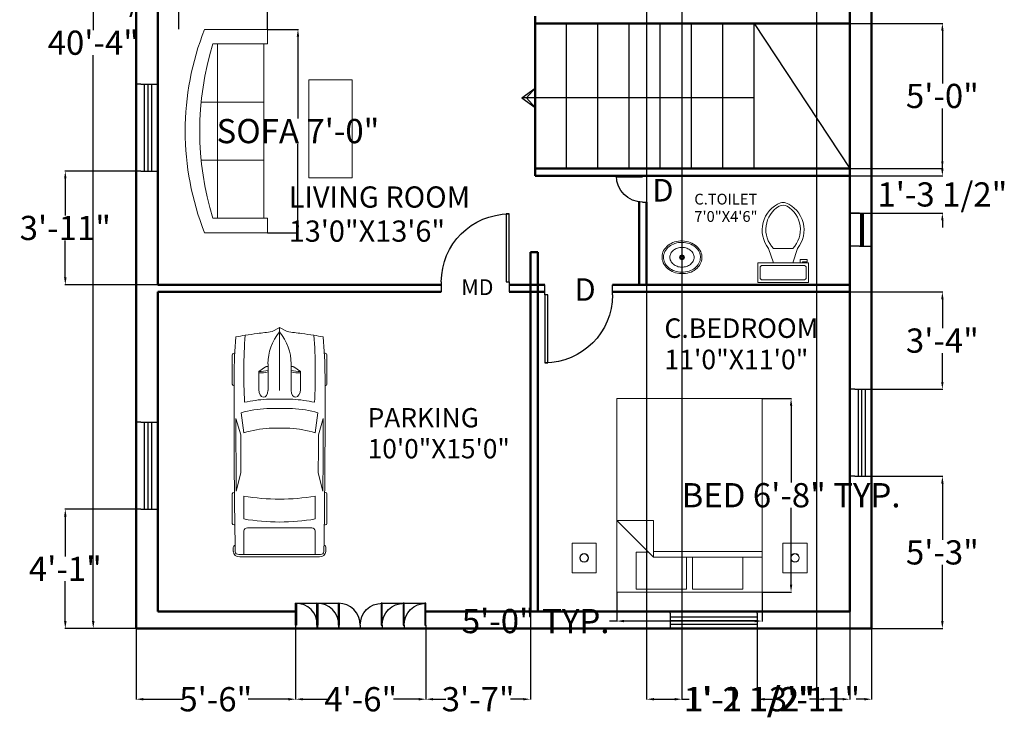
# Model space of a CAD drawing. Units: inches. Extents: x -35 to 382, y 867 to 1468.
# Tile 1 of 3: x -35 to 372, y 867 to 1163. Entities that reach past the tile are written whole.
import ezdxf

# ---------------------------------------------------------------- set-up
doc = ezdxf.new("R2010")
doc.units = ezdxf.units.IN
doc.header["$MEASUREMENT"] = 0
for name, color, linetype, lineweight in [('A-ANNO-DIMS', 2, 'Continuous', 18), ('A-ANNO-TEXT', 7, 'Continuous', 25), ('A-AREA-IDEN', 7, 'Continuous', 25), ('A-DOOR', 3, 'Continuous', 25), ('A-FLOR-FIXT', 9, 'Continuous', 18), ('A-FLOR-STRS', 7, 'Continuous', 25), ('A-FURN', 9, 'Continuous', 18), ('A-GLAZ', 4, 'Continuous', 25), ('A-SITE-VEHC', 8, 'Continuous', 13), ('A-WALL', 7, 'Continuous', 50)]:
    doc.layers.add(name, color=color, linetype=linetype, lineweight=lineweight)
doc.styles.get("Standard").update_dxf_attribs({"font": 'arial.ttf'})
doc.dimstyles.get("Standard").update_dxf_attribs({"dimtxt": 10, "dimasz": 3, "dimexe": 0.18, "dimexo": 0.0625, "dimgap": 0.09, "dimtad": 0, "dimtih": 1, "dimtoh": 1, "dimdec": 0, "dimzin": 0, "dimdsep": 46, "dimlunit": 3, "dimtxsty": 'Standard', "dimcen": 0.09, "dimadec": 0, "dimazin": 0, "dimtfac": 1, "dimtdec": 0, "dimtofl": 0, "dimtmove": 0, "dimatfit": 3, "dimfxl": 1, "dimtolj": 1, "dimtzin": 0, "dimarcsym": 0})

# ---------------------------------------------------------------- blocks, each defined once
blk = doc.blocks.new('Sofa - Roundback 7 ft.')
for p, q in [((-12.00002, -32.4421), (-12.00003, -6.5971)), ((11.99997, -32.4421), (11.99998, -6.5971)), ((-36.000027, -34), (-36.000027, -11.4696)), ((35.99998, -34), (35.99998, -11.4696)), ((-35.999844, -13.3819), (35.9998, -13.3819)), ((-36.000027, -32.4421), (35.99998, -32.4421))]:
    blk.add_line(p, q)
for points in [[(-36.000027, -34), (-42.000027, -34), (-42.000027, -8)], [(41.99998, -8), (41.99998, -34), (35.99998, -34)]]:
    blk.add_lwpolyline(points)
for centre, radius, start, end in [((0, -114.25), 114.25, 68.43141, 111.5686), ((-0.00001, -127.1968), 121.1968, 72.72033, 107.2797)]:
    blk.add_arc(centre, radius, start, end)
blk = doc.blocks.new('*U11')
for p, q in [((536, 950), (536, 936)), ((1182, 988), (568, 988)), ((1214, 950), (1214, 950)), ((2235, 810), (1899, 912)), ((3412, 904), (3030, 807)), ((3440, 942), (3440, 950)), ((3472, 988), (4087, 988)), ((4119, 950), (4119, 934)), ((4736, -851), (4736, 851)), ((4785, -832), (4785, 832)), ((1779, 801), (2195, 746)), ((3516, 746), (3994, 746)), ((4179, 670), (4179, -670)), ((4736, 746), (4242, 746)), ((820, 295), (918, 436)), ((918, 436), (1294, 436)), ((756, 241), (1313, 241)), ((816, 241), (816, 283)), ((1496, -274), (1496, 274)), ((1690, -267), (1690, 267)), ((2102, 216), (2102, -216)), ((4736, -267), (4736, 267)), ((83, 156), (3, 10)), ((0, 0), (1313, 0)), ((3, -10), (83, -156)), ((756, -241), (1313, -241)), ((816, -241), (816, -283)), ((820, -295), (918, -436)), ((918, -436), (1294, -436)), ((2195, -746), (1779, -801)), ((2235, -810), (1899, -912)), ((3412, -904), (3030, -807)), ((3994, -746), (3516, -746)), ((4242, -746), (4736, -746)), ((536, -950), (536, -936)), ((1182, -988), (568, -988)), ((1214, -950), (1214, -950)), ((3440, -942), (3440, -950)), ((3472, -988), (4087, -988)), ((4119, -950), (4119, -934))]:
    blk.add_line(p, q)
for centre, major_axis, ratio, start_param, end_param in [((6757, -699), (0, 7958), 0.842304, 1.367076, 1.39176), ((1046, -12468), (0, 13417), 0.842304, 0.00281, 0.075598), ((568, 950), (0, -37.6), 0.842304, 3.141593, 4.712389), ((1638, -268113), (0, 269063), 0.842304, -0.013397, 0.002797), ((1182, 950), (0, 37.6), 0.842304, -1.570796, 0), ((1638, -268113), (0, -269025), 0.842304, 3.133765, 3.140441), ((3472, 950), (0, -37.6), 0.842304, 3.141593, 4.712389), ((4087, 950), (0, 37.6), 0.842304, -1.570796, 0), ((4588, 910), (0, 56.4), 0.842304, -0.013017, 1.249894), ((1638, -268131), (0, 269121), 0.842304, -0.013397, -0.013017), ((4673, 851), (0, -75.2), 0.842304, 1.570796, 3.128196), ((4673, 832), (0, -133), 0.842304, 1.570796, 3.128196), ((6583, -699), (0, -7755), 0.842304, 4.528606, 4.561838), ((952, -15087), (0, -15833), 0.842304, 3.096046, 3.200911), ((3414, 137), (0, -2280), 0.842304, 4.449482, 4.652344), ((3436, 137), (0, 2077), 0.842304, 1.245306, 1.50788), ((3800, 71), (0, -2021), 0.842304, 4.372215, 4.640744), ((2433, -93125), (0, -93935), 0.842304, 3.134049, 3.144098), ((434, 0), (0, 3734), 0.842304, 4.511394, 4.913384), ((912, 0), (0, 3734), 0.842304, 4.511394, 4.913384), ((4242, 670), (0, 75.2), 0.842304, 0, 1.570796), ((-5194, 1331), (0, -6374), 0.842304, 1.385369, 1.434372), ((331, 432), (0, 696), 0.842304, 4.435146, 4.718221), ((361, 432), (0, 696), 0.842304, 4.435146, 4.718221), ((1290, 339), (161, -9), 0.603834, -1.395552, 1.581315), ((756, -1185), (0, 1427), 0.842304, 0, 0.590319), ((832, 283), (0, 18.8), 0.842304, 0.879714, 1.570796), ((16, 0), (0, -18.8), 0.842304, 4.131459, 5.293319), ((-5194, -1331), (0, 6374), 0.842304, -1.434372, -1.385369), ((756, 1185), (0, 1427), 0.842304, 2.551274, 3.141593), ((832, -283), (0, -18.8), 0.842304, 4.712389, 5.403472), ((331, -432), (0, -696), 0.842304, 1.564964, 1.848039), ((361, -432), (0, -696), 0.842304, 1.564964, 1.848039), ((3414, -137), (0, -2280), 0.842304, -1.510751, -1.307889), ((3436, -137), (0, -2077), 0.842304, -1.50788, -1.245306), ((3800, -71), (0, -2021), 0.842304, -1.499151, -1.230623), ((6583, 699), (0, 7755), 0.842304, 1.721348, 1.754579), ((6757, 699), (0, 7958), 0.842304, 1.749832, 1.774517), ((952, 15087), (0, -15833), 0.842304, -0.059319, 0.045547), ((2433, 93125), (0, -93935), 0.842304, -0.002505, 0.007544), ((4242, -670), (0, -75.2), 0.842304, 4.712389, 6.283185), ((1046, 12468), (0, -13417), 0.842304, -0.075598, -0.00281), ((568, -950), (0, 37.6), 0.842304, 1.570796, 3.141593), ((1638, 268113), (0, 269063), 0.842304, 3.138796, 3.15499), ((1182, -950), (0, -37.6), 0.842304, 0, 1.570796), ((1638, 268113), (0, -269025), 0.842304, 0.001152, 0.007828), ((3472, -950), (0, -37.6), 0.842304, -1.570796, 0), ((4087, -950), (0, 37.6), 0.842304, 3.141593, 4.712389), ((4588, -910), (0, -56.4), 0.842304, -1.249894, 0.013017), ((1638, 268131), (0, 269121), 0.842304, 3.15461, 3.15499), ((4673, -851), (0, 75.2), 0.842304, 3.15499, 4.712389), ((4673, -832), (0, -133), 0.842304, 0.013397, 1.570796)]:
    blk.add_ellipse(centre, major_axis=major_axis, ratio=ratio, start_param=start_param, end_param=end_param)
at = {"extrusion": (0, 0, -1)}
blk.add_ellipse((1290, -339), major_axis=(161, 9), ratio=0.603834, start_param=-1.395552, end_param=1.581315, dxfattribs=at)
blk = doc.blocks.new('*U9')
for p, q in [((0, 0), (0, -6)), ((40, 0), (40, -6))]:
    blk.add_line(p, q)
blk.add_lwpolyline([(0, 0), (0, 40), (1.75, 40), (1.75, 0)], close=True)
blk.add_arc((0, 0), 40, 0, 90)
blk = doc.blocks.new('Bed - Queen')
for p, q in [((0, -80.00003), (0, 0)), ((0, 0), (59.99999, 0)), ((59.99999, 0), (59.99999, -80.00003)), ((7.99999, -1.2), (28.79998, -1.2)), ((7.99999, -14.4), (7.99999, -1.2)), ((28.79998, -1.2), (28.79998, -14.4)), ((31.19999, -1.2), (51.99999, -1.2)), ((31.19999, -14.4), (31.19999, -1.2)), ((51.99999, -1.2), (51.99999, -16.4)), ((0, -14.4), (44.8, -14.4)), ((59.99999, -29.6), (44.8, -14.4)), ((44.8, -14.4), (44.8, -29.6)), ((44.8, -16.8), (0, -16.8)), ((51.99999, -16.4), (46.79936, -16.4)), ((44.8, -29.6), (59.99999, -29.6)), ((59.99999, -80.00003), (0, -80.00003))]:
    blk.add_line(p, q)
blk = doc.blocks.new('Sink - Oval top')
for p, q in [((-1, 0), (1, 0)), ((0, 1), (0, -1))]:
    blk.add_line(p, q)
for points in [[(-12.23, 0.39, 0.117634), (-11.46, -3.36, 0.104469), (-8.88, -6.8, 0.090016), (-5.08, -9.07, 0.08192), (-0.32, -10.02, 0.08192), (4.49, -9.38, 0.090016), (8.42, -7.36, 0.104469), (11.22, -4.09, 0.117634), (12.23, -0.39, 0.117634), (11.46, 3.36, 0.104469), (8.88, 6.8, 0.090016), (5.08, 9.07, 0.08192), (0.32, 10.02, 0.08192), (-4.49, 9.38, 0.090016), (-8.42, 7.36, 0.104469), (-11.22, 4.09, 0.117634)], [(-11.29, 0.16, 0.118622), (-10.52, -3.25, 0.104678), (-8.07, -6.36, 0.089562), (-4.54, -8.37, 0.081185), (-0.13, -9.15, 0.081185), (4.3, -8.49, 0.089562), (7.89, -6.58, 0.104678), (10.42, -3.55, 0.118622), (11.29, -0.16, 0.118622), (10.52, 3.25, 0.104678), (8.07, 6.36, 0.089562), (4.54, 8.37, 0.081185), (0.13, 9.15, 0.081185), (-4.3, 8.49, 0.089562), (-7.89, 6.58, 0.104678), (-10.42, 3.55, 0.118622)], [(-7.42, 0.08, 0.118283), (-6.91, -2.17, 0.104607), (-5.29, -4.21, 0.089718), (-2.97, -5.53, 0.081436), (-0.07, -6.04, 0.081436), (2.84, -5.59, 0.089718), (5.2, -4.33, 0.104607), (6.86, -2.32, 0.118283), (7.42, -0.08, 0.118283), (6.91, 2.17, 0.104607), (5.29, 4.21, 0.089718), (2.97, 5.53, 0.081436), (0.07, 6.04, 0.081436), (-2.84, 5.59, 0.089718), (-5.2, 4.33, 0.104607), (-6.86, 2.32, 0.118283)]]:
    blk.add_lwpolyline(points, format="xyb", close=True)
for radius in [1.5, 1]:
    blk.add_circle((0, 0), radius)
blk = doc.blocks.new('Toilet - top')
for p, q in [((9.5, -6), (9.5, -2)), ((-8, -8.5), (-8, -8)), ((-7, -8), (-7, -9.5)), ((-4, -8), (-6, -14)), ((4, -8), (6, -14)), ((-10, -8.5), (-8, -8.5)), ((-10, -9.5), (-10, -8.5)), ((-7, -9.5), (-10, -9.5)), ((4, -14), (-4, -14))]:
    blk.add_line(p, q)
blk.add_lwpolyline([(10.5, -8), (10.5, 0), (-10.5, 0), (-10.5, -8)], close=True)
for points in [[(-9.5, -2), (-9.5, -6)], [(8.5, -1), (-8.5, -1)], [(-8.5, -7), (8.5, -7)]]:
    blk.add_lwpolyline(points)
for centre, radius, start, end in [((-8.62, -1.88), 0.884, 81.8699, 188.1301), ((8.62, -1.88), 0.884, 351.8699, 98.1301), ((-8.62, -6.12), 0.884, 171.8699, 278.1301), ((8.62, -6.12), 0.884, 261.8699, 8.1301), ((3.52, -21.58), 12.17, 141.4691, 247.9714), ((4.2, -21.82), 11.33, 136.3677, 238.9468), ((-3.52, -21.58), 12.17, 292.0284, 38.5307), ((-4.2, -21.82), 11.33, 301.053, 43.6321), ((0, -27.88), 4, 245.7318, 294.2682), ((0, -29), 4, 254.8605, 285.1395)]:
    blk.add_arc(centre, radius, start, end)
blk = doc.blocks.new('Window - Wood Frame 36 in. Wide plan')
for p, q in [((0, 6), (0, 0)), ((0, 4.5), (36, 4.5)), ((36, 6), (36, 0)), ((0, 3), (36, 3)), ((0, 1.5), (36, 1.5))]:
    blk.add_line(p, q)
blk = doc.blocks.new('*D16')
at = {"layer": 'A-ANNO-DIMS', "color": 0, "lineweight": -2, "transparency": 16777216}
for p, q in [((13.46, 1395.31), (-4.36, 1395.31)), ((-4.18, 1392.31), (-4.18, 1158.51)), ((-4.18, 914.31), (-4.18, 1148.12)), ((13.46, 911.31), (-4.36, 911.31))]:
    blk.add_line(p, q, dxfattribs=at)
at = {"layer": 'A-ANNO-DIMS', "color": 0, "transparency": 16777216}
for points in [[(-4.68, 1392.31), (-3.68, 1392.31), (-4.18, 1395.31)], [(-4.68, 914.31), (-3.68, 914.31), (-4.18, 911.31)]]:
    blk.add_solid(points, dxfattribs=at)
at = {"layer": 'Defpoints', "color": 0, "transparency": 16777216}
for p in [(13.52, 1395.31), (-4.18, 911.31), (13.52, 911.31)]:
    blk.add_point(p, dxfattribs=at)
at = {"layer": 'A-ANNO-DIMS', "color": 0, "transparency": 16777216, "insert": (-4.18, 1153.31), "char_height": 10, "attachment_point": 5}
blk.add_mtext('\\A1;40\'-4"', dxfattribs=at)
blk = doc.blocks.new('BEDSIDE-TABLE')
blk.add_lwpolyline([(0, 12.34), (9.96, 12.34), (9.96, 0), (0, 0)], close=True)
for radius in [1.78, 1.78, 1.66]:
    blk.add_circle((4.98, 6.17), radius)
blk = doc.blocks.new('*D24')
at = {"layer": 'A-ANNO-DIMS', "color": 0, "lineweight": -2, "transparency": 16777216}
for p, q in [((272.3, 1006.35), (284.42, 1006.35)), ((284.24, 1003.35), (284.24, 971.55)), ((284.24, 929.35), (284.24, 961.16)), ((272.3, 926.35), (284.42, 926.35))]:
    blk.add_line(p, q, dxfattribs=at)
at = {"layer": 'A-ANNO-DIMS', "color": 0, "transparency": 16777216}
for points in [[(283.74, 1003.35), (284.74, 1003.35), (284.24, 1006.35)], [(283.74, 929.35), (284.74, 929.35), (284.24, 926.35)]]:
    blk.add_solid(points, dxfattribs=at)
at = {"layer": 'Defpoints', "color": 0, "transparency": 16777216}
for p in [(272.24, 1006.35), (272.24, 926.35), (284.24, 926.35)]:
    blk.add_point(p, dxfattribs=at)
at = {"layer": 'A-ANNO-DIMS', "color": 0, "transparency": 16777216, "insert": (284.24, 966.35), "char_height": 10, "attachment_point": 5}
blk.add_mtext('\\A1;BED 6\'-8" TYP.', dxfattribs=at)
blk = doc.blocks.new('*D25')
at = {"layer": 'A-ANNO-DIMS', "color": 0, "lineweight": -2, "transparency": 16777216}
for p, q in [((212.24, 926.29), (212.24, 914.17)), ((272.24, 926.29), (272.24, 914.17)), ((212.24, 914.35), (209.24, 914.35)), ((269.24, 914.35), (215.24, 914.35))]:
    blk.add_line(p, q, dxfattribs=at)
at = {"layer": 'A-ANNO-DIMS', "color": 0, "transparency": 16777216}
for points in [[(215.24, 914.85), (215.24, 913.85), (212.24, 914.35)], [(269.24, 914.85), (269.24, 913.85), (272.24, 914.35)]]:
    blk.add_solid(points, dxfattribs=at)
at = {"layer": 'Defpoints', "color": 0, "transparency": 16777216}
for p in [(212.24, 926.35), (272.24, 926.35), (212.24, 914.35)]:
    blk.add_point(p, dxfattribs=at)
at = {"layer": 'A-ANNO-DIMS', "color": 0, "transparency": 16777216, "insert": (178.67, 914.35), "char_height": 10, "attachment_point": 5}
blk.add_mtext('\\A1;5\'-0" TYP.', dxfattribs=at)
blk = doc.blocks.new('*D30')
at = {"layer": 'A-ANNO-DIMS', "color": 0, "lineweight": -2, "transparency": 16777216}
for p, q in [((67.88, 1158.79), (80.6, 1158.79)), ((80.42, 1155.79), (80.42, 1122.05)), ((80.42, 1077.79), (80.42, 1111.52)), ((67.88, 1074.79), (80.6, 1074.79))]:
    blk.add_line(p, q, dxfattribs=at)
at = {"layer": 'A-ANNO-DIMS', "color": 0, "transparency": 16777216}
for points in [[(79.92, 1155.79), (80.92, 1155.79), (80.42, 1158.79)], [(79.92, 1077.79), (80.92, 1077.79), (80.42, 1074.79)]]:
    blk.add_solid(points, dxfattribs=at)
at = {"layer": 'Defpoints', "color": 0, "transparency": 16777216}
for p in [(67.82, 1158.79), (80.42, 1158.79), (67.82, 1074.79)]:
    blk.add_point(p, dxfattribs=at)
at = {"layer": 'A-ANNO-DIMS', "color": 0, "transparency": 16777216, "insert": (80.42, 1116.79), "char_height": 10, "attachment_point": 5}
blk.add_mtext('\\A1;SOFA 7\'-0"', dxfattribs=at)
blk = doc.blocks.new('*D31')
at = {"layer": 'A-ANNO-DIMS', "color": 0, "lineweight": -2, "transparency": 16777216}
for p, q in [((31.15, 1171.39), (28.15, 1171.39)), ((31.15, 1158.85), (31.15, 1171.57)), ((64.82, 1171.39), (34.15, 1171.39)), ((67.82, 1158.85), (67.82, 1171.57))]:
    blk.add_line(p, q, dxfattribs=at)
at = {"layer": 'A-ANNO-DIMS', "color": 0, "transparency": 16777216}
for points in [[(34.15, 1171.89), (34.15, 1170.89), (31.15, 1171.39)], [(64.82, 1171.89), (64.82, 1170.89), (67.82, 1171.39)]]:
    blk.add_solid(points, dxfattribs=at)
at = {"layer": 'Defpoints', "color": 0, "transparency": 16777216}
for p in [(31.15, 1171.39), (31.15, 1158.79), (67.82, 1158.79)]:
    blk.add_point(p, dxfattribs=at)
at = {"layer": 'A-ANNO-DIMS', "color": 0, "transparency": 16777216, "insert": (3.12, 1171.39), "char_height": 10, "attachment_point": 5}
blk.add_mtext('\\A1;3\'-0 1/2"', dxfattribs=at)
blk = doc.blocks.new('*D36')
at = {"layer": 'A-ANNO-DIMS', "color": 0, "lineweight": -2, "transparency": 16777216}
for p, q in [((87.91, 1187.13), (87.91, 1173.36)), ((178.91, 1187.13), (178.91, 1173.36)), ((90.91, 1173.54), (175.91, 1173.54)), ((178.91, 1173.54), (181.91, 1173.54))]:
    blk.add_line(p, q, dxfattribs=at)
at = {"layer": 'A-ANNO-DIMS', "color": 0, "transparency": 16777216}
for points in [[(90.91, 1174.04), (90.91, 1173.04), (87.91, 1173.54)], [(175.91, 1174.04), (175.91, 1173.04), (178.91, 1173.54)]]:
    blk.add_solid(points, dxfattribs=at)
at = {"layer": 'Defpoints', "color": 0, "transparency": 16777216}
for p in [(87.91, 1187.19), (178.91, 1187.19), (178.91, 1173.54)]:
    blk.add_point(p, dxfattribs=at)
at = {"layer": 'A-ANNO-DIMS', "color": 0, "transparency": 16777216, "insert": (236.96, 1173.54), "char_height": 10, "attachment_point": 5}
blk.add_mtext('\\A1;DINING SET 7\'-7"', dxfattribs=at)
blk = doc.blocks.new('*D38')
at = {"layer": 'A-ANNO-DIMS', "color": 0, "lineweight": -2, "transparency": 16777216}
for p, q in [((13.52, 911.25), (13.52, 881.88)), ((79.43, 911.25), (79.43, 881.88)), ((16.52, 882.06), (33.09, 882.06)), ((76.43, 882.06), (59.86, 882.06))]:
    blk.add_line(p, q, dxfattribs=at)
at = {"layer": 'A-ANNO-DIMS', "color": 0, "transparency": 16777216}
for points in [[(16.52, 882.56), (16.52, 881.56), (13.52, 882.06)], [(76.43, 882.56), (76.43, 881.56), (79.43, 882.06)]]:
    blk.add_solid(points, dxfattribs=at)
at = {"layer": 'Defpoints', "color": 0, "transparency": 16777216}
for p in [(13.52, 911.31), (79.43, 911.31), (79.43, 882.06)]:
    blk.add_point(p, dxfattribs=at)
at = {"layer": 'A-ANNO-DIMS', "color": 0, "transparency": 16777216, "insert": (46.47, 882.06), "char_height": 10, "attachment_point": 5}
blk.add_mtext('\\A1;5\'-6"', dxfattribs=at)
blk = doc.blocks.new('*D39')
at = {"layer": 'A-ANNO-DIMS', "color": 0, "lineweight": -2, "transparency": 16777216}
for p, q in [((79.43, 911.25), (79.43, 881.88)), ((133.31, 911.25), (133.31, 881.88)), ((82.43, 882.06), (92.78, 882.06)), ((130.31, 882.06), (119.95, 882.06))]:
    blk.add_line(p, q, dxfattribs=at)
at = {"layer": 'A-ANNO-DIMS', "color": 0, "transparency": 16777216}
for points in [[(82.43, 882.56), (82.43, 881.56), (79.43, 882.06)], [(130.31, 882.56), (130.31, 881.56), (133.31, 882.06)]]:
    blk.add_solid(points, dxfattribs=at)
at = {"layer": 'Defpoints', "color": 0, "transparency": 16777216}
for p in [(79.43, 911.31), (133.31, 911.31), (133.31, 882.06)]:
    blk.add_point(p, dxfattribs=at)
at = {"layer": 'A-ANNO-DIMS', "color": 0, "transparency": 16777216, "insert": (106.37, 882.06), "char_height": 10, "attachment_point": 5}
blk.add_mtext('\\A1;4\'-6"', dxfattribs=at)
blk = doc.blocks.new('*D40')
at = {"layer": 'A-ANNO-DIMS', "color": 0, "lineweight": -2, "transparency": 16777216}
for p, q in [((176.52, 918.25), (176.52, 881.88)), ((133.31, 911.25), (133.31, 881.88)), ((136.31, 882.06), (141.54, 882.06)), ((173.52, 882.06), (168.29, 882.06))]:
    blk.add_line(p, q, dxfattribs=at)
at = {"layer": 'A-ANNO-DIMS', "color": 0, "transparency": 16777216}
for points in [[(136.31, 882.56), (136.31, 881.56), (133.31, 882.06)], [(173.52, 882.56), (173.52, 881.56), (176.52, 882.06)]]:
    blk.add_solid(points, dxfattribs=at)
at = {"layer": 'Defpoints', "color": 0, "transparency": 16777216}
for p in [(176.52, 918.31), (133.31, 911.31), (176.52, 882.06)]:
    blk.add_point(p, dxfattribs=at)
at = {"layer": 'A-ANNO-DIMS', "color": 0, "transparency": 16777216, "insert": (154.91, 882.06), "char_height": 10, "attachment_point": 5}
blk.add_mtext('\\A1;3\'-7"', dxfattribs=at)
blk = doc.blocks.new('*D41')
at = {"layer": 'A-ANNO-DIMS', "color": 0, "lineweight": -2, "transparency": 16777216}
for p, q in [((270.28, 911.51), (270.28, 881.88)), ((317.52, 911.25), (317.52, 881.88)), ((273.28, 882.06), (276.64, 882.06)), ((314.52, 882.06), (311.17, 882.06))]:
    blk.add_line(p, q, dxfattribs=at)
at = {"layer": 'A-ANNO-DIMS', "color": 0, "transparency": 16777216}
for points in [[(273.28, 882.56), (273.28, 881.56), (270.28, 882.06)], [(314.52, 882.56), (314.52, 881.56), (317.52, 882.06)]]:
    blk.add_solid(points, dxfattribs=at)
at = {"layer": 'Defpoints', "color": 0, "transparency": 16777216}
for p in [(270.28, 911.57), (317.52, 911.31), (270.28, 882.06)]:
    blk.add_point(p, dxfattribs=at)
at = {"layer": 'A-ANNO-DIMS', "color": 0, "transparency": 16777216, "insert": (293.9, 882.06), "char_height": 10, "attachment_point": 5}
blk.add_mtext('\\A1;3\'-11"', dxfattribs=at)
blk = doc.blocks.new('*D42')
at = {"layer": 'A-ANNO-DIMS', "color": 0, "lineweight": -2, "transparency": 16777216}
for p, q in [((308.58, 1050.31), (346.95, 1050.31)), ((346.77, 1047.31), (346.77, 1035.43)), ((346.77, 1013.15), (346.77, 1025.03)), ((317.58, 1010.15), (346.95, 1010.15))]:
    blk.add_line(p, q, dxfattribs=at)
at = {"layer": 'A-ANNO-DIMS', "color": 0, "transparency": 16777216}
for points in [[(346.27, 1047.31), (347.27, 1047.31), (346.77, 1050.31)], [(346.27, 1013.15), (347.27, 1013.15), (346.77, 1010.15)]]:
    blk.add_solid(points, dxfattribs=at)
at = {"layer": 'Defpoints', "color": 0, "transparency": 16777216}
for p in [(308.52, 1050.31), (346.77, 1050.31), (317.52, 1010.15)]:
    blk.add_point(p, dxfattribs=at)
at = {"layer": 'A-ANNO-DIMS', "color": 0, "transparency": 16777216, "insert": (346.77, 1030.23), "char_height": 10, "attachment_point": 5}
blk.add_mtext('\\A1;3\'-4"', dxfattribs=at)
blk = doc.blocks.new('*D44')
at = {"layer": 'A-ANNO-DIMS', "color": 0, "lineweight": -2, "transparency": 16777216}
for p, q in [((308.58, 1161.31), (346.95, 1161.31)), ((346.77, 1158.31), (346.77, 1136.51)), ((346.77, 1104.31), (346.77, 1126.12)), ((308.58, 1101.31), (346.95, 1101.31))]:
    blk.add_line(p, q, dxfattribs=at)
at = {"layer": 'A-ANNO-DIMS', "color": 0, "transparency": 16777216}
for points in [[(346.27, 1158.31), (347.27, 1158.31), (346.77, 1161.31)], [(346.27, 1104.31), (347.27, 1104.31), (346.77, 1101.31)]]:
    blk.add_solid(points, dxfattribs=at)
at = {"layer": 'Defpoints', "color": 0, "transparency": 16777216}
for p in [(308.52, 1161.31), (346.77, 1161.31), (308.52, 1101.31)]:
    blk.add_point(p, dxfattribs=at)
at = {"layer": 'A-ANNO-DIMS', "color": 0, "transparency": 16777216, "insert": (346.77, 1131.31), "char_height": 10, "attachment_point": 5}
blk.add_mtext('\\A1;5\'-0"', dxfattribs=at)
blk = doc.blocks.new('*D45')
at = {"layer": 'A-ANNO-DIMS', "color": 0, "lineweight": -2, "transparency": 16777216}
for p, q in [((239.15, 1224.59), (239.15, 881.88)), ((224.52, 1215.25), (224.52, 881.88)), ((227.52, 882.06), (236.15, 882.06)), ((239.15, 882.06), (242.15, 882.06))]:
    blk.add_line(p, q, dxfattribs=at)
at = {"layer": 'A-ANNO-DIMS', "color": 0, "transparency": 16777216}
for points in [[(227.52, 882.56), (227.52, 881.56), (224.52, 882.06)], [(236.15, 882.56), (236.15, 881.56), (239.15, 882.06)]]:
    blk.add_solid(points, dxfattribs=at)
at = {"layer": 'Defpoints', "color": 0, "transparency": 16777216}
for p in [(239.15, 1224.65), (224.52, 1215.31), (239.15, 882.06)]:
    blk.add_point(p, dxfattribs=at)
at = {"layer": 'A-ANNO-DIMS', "color": 0, "transparency": 16777216, "insert": (266.71, 882.06), "char_height": 10, "attachment_point": 5}
blk.add_mtext('\\A1;1\'-2 1/2"', dxfattribs=at)
blk = doc.blocks.new('*D46')
at = {"layer": 'A-ANNO-DIMS', "color": 0, "lineweight": -2, "transparency": 16777216}
for p, q in [((294.81, 1215.25), (294.81, 881.88)), ((308.52, 1215.25), (308.52, 881.88)), ((294.81, 882.06), (291.81, 882.06)), ((305.52, 882.06), (297.81, 882.06))]:
    blk.add_line(p, q, dxfattribs=at)
at = {"layer": 'A-ANNO-DIMS', "color": 0, "transparency": 16777216}
for points in [[(297.81, 882.56), (297.81, 881.56), (294.81, 882.06)], [(305.52, 882.56), (305.52, 881.56), (308.52, 882.06)]]:
    blk.add_solid(points, dxfattribs=at)
at = {"layer": 'Defpoints', "color": 0, "transparency": 16777216}
for p in [(294.81, 1215.31), (308.52, 1215.31), (294.81, 882.06)]:
    blk.add_point(p, dxfattribs=at)
at = {"layer": 'A-ANNO-DIMS', "color": 0, "transparency": 16777216, "insert": (267.25, 882.06), "char_height": 10, "attachment_point": 5}
blk.add_mtext('\\A1;1\'-1 1/2"', dxfattribs=at)
blk = doc.blocks.new('*D50')
at = {"layer": 'A-ANNO-DIMS', "color": 0, "lineweight": -2, "transparency": 16777216}
for p, q in [((317.58, 974.15), (346.95, 974.15)), ((346.77, 971.15), (346.77, 947.93)), ((346.77, 914.31), (346.77, 937.53)), ((317.58, 911.31), (346.95, 911.31))]:
    blk.add_line(p, q, dxfattribs=at)
at = {"layer": 'A-ANNO-DIMS', "color": 0, "transparency": 16777216}
for points in [[(346.27, 971.15), (347.27, 971.15), (346.77, 974.15)], [(346.27, 914.31), (347.27, 914.31), (346.77, 911.31)]]:
    blk.add_solid(points, dxfattribs=at)
at = {"layer": 'Defpoints', "color": 0, "transparency": 16777216}
for p in [(317.52, 974.15), (346.77, 974.15), (317.52, 911.31)]:
    blk.add_point(p, dxfattribs=at)
at = {"layer": 'A-ANNO-DIMS', "color": 0, "transparency": 16777216, "insert": (346.77, 942.73), "char_height": 10, "attachment_point": 5}
blk.add_mtext('\\A1;5\'-3"', dxfattribs=at)
blk = doc.blocks.new('*D51')
at = {"layer": 'A-ANNO-DIMS', "color": 0, "lineweight": -2, "transparency": 16777216}
for p, q in [((13.46, 960.55), (-15.91, 960.55)), ((-15.73, 957.55), (-15.73, 941.04)), ((-15.73, 914.31), (-15.73, 930.82)), ((13.46, 911.31), (-15.91, 911.31))]:
    blk.add_line(p, q, dxfattribs=at)
at = {"layer": 'A-ANNO-DIMS', "color": 0, "transparency": 16777216}
for points in [[(-16.23, 957.55), (-15.23, 957.55), (-15.73, 960.55)], [(-16.23, 914.31), (-15.23, 914.31), (-15.73, 911.31)]]:
    blk.add_solid(points, dxfattribs=at)
at = {"layer": 'Defpoints', "color": 0, "transparency": 16777216}
for p in [(-15.73, 960.55), (13.52, 960.55), (13.52, 911.31)]:
    blk.add_point(p, dxfattribs=at)
at = {"layer": 'A-ANNO-DIMS', "color": 0, "transparency": 16777216, "insert": (-15.73, 935.93), "char_height": 10, "attachment_point": 5}
blk.add_mtext('\\A1;4\'-1"', dxfattribs=at)
blk = doc.blocks.new('*D52')
at = {"layer": 'A-ANNO-DIMS', "color": 0, "lineweight": -2, "transparency": 16777216}
for p, q in [((13.46, 1100.23), (-15.91, 1100.23)), ((-15.73, 1097.23), (-15.73, 1081.97)), ((-15.73, 1056.31), (-15.73, 1071.57)), ((22.46, 1053.31), (-15.91, 1053.31))]:
    blk.add_line(p, q, dxfattribs=at)
at = {"layer": 'A-ANNO-DIMS', "color": 0, "transparency": 16777216}
for points in [[(-16.23, 1097.23), (-15.23, 1097.23), (-15.73, 1100.23)], [(-16.23, 1056.31), (-15.23, 1056.31), (-15.73, 1053.31)]]:
    blk.add_solid(points, dxfattribs=at)
at = {"layer": 'Defpoints', "color": 0, "transparency": 16777216}
for p in [(-15.73, 1100.23), (13.52, 1100.23), (22.52, 1053.31)]:
    blk.add_point(p, dxfattribs=at)
at = {"layer": 'A-ANNO-DIMS', "color": 0, "transparency": 16777216, "insert": (-15.73, 1076.77), "char_height": 10, "attachment_point": 5}
blk.add_mtext('\\A1;3\'-11"', dxfattribs=at)
blk = doc.blocks.new('*D54')
at = {"layer": 'A-ANNO-DIMS', "color": 0, "lineweight": -2, "transparency": 16777216}
for p, q in [((346.771307, 1101.314909), (346.771307, 1104.314909)), ((308.583807, 1098.314909), (346.951307, 1098.314909)), ((308.583807, 1082.911631), (346.951307, 1082.911631)), ((346.771307, 1079.911631), (346.771307, 1076.911631))]:
    blk.add_line(p, q, dxfattribs=at)
at = {"layer": 'A-ANNO-DIMS', "color": 0, "transparency": 16777216}
for points in [[(346.271307, 1101.314909), (347.271307, 1101.314909), (346.771307, 1098.314909)], [(346.271307, 1079.911631), (347.271307, 1079.911631), (346.771307, 1082.911631)]]:
    blk.add_solid(points, dxfattribs=at)
at = {"layer": 'Defpoints', "color": 0, "transparency": 16777216}
for p in [(308.521307, 1098.314909), (308.521307, 1082.911631), (346.771307, 1082.911631)]:
    blk.add_point(p, dxfattribs=at)
at = {"layer": 'A-ANNO-DIMS', "color": 0, "transparency": 16777216, "insert": (346.771307, 1090.61327), "char_height": 10, "attachment_point": 5}
blk.add_mtext('\\A1;1\'-3 1/2"', dxfattribs=at)

msp = doc.modelspace()

# ---------------------------------------------------------------- linework, layer by layer
at = {"layer": 'A-DOOR'}
for p, q in [((79.43, 921.72), (88.28, 921.72)), ((88.28, 921.72), (97.12, 921.72)), ((115.22, 921.72), (124.26, 921.72)), ((124.26, 921.72), (133.31, 921.72))]:
    msp.add_line(p, q, dxfattribs=at)
at = {"layer": 'A-FLOR-STRS'}
for p, q in [((178.52, 1101.31), (178.52, 1161.31)), ((191.44, 1101.31), (191.44, 1161.31)), ((204.36, 1101.31), (204.36, 1161.31)), ((217.28, 1101.31), (217.28, 1161.31)), ((230.2, 1101.31), (230.2, 1161.31)), ((243.12, 1101.31), (243.12, 1161.31)), ((256.04, 1101.31), (256.04, 1161.31)), ((268.96, 1101.31), (268.96, 1161.31)), ((268.96, 1161.31), (308.52, 1101.31)), ((173.02, 1130.47), (178.52, 1134.47)), ((178.52, 1134.47), (174.91, 1130.47)), ((268.96, 1130.47), (173.02, 1130.47)), ((173.02, 1130.47), (178.52, 1126.48)), ((178.52, 1126.48), (174.91, 1130.47))]:
    msp.add_line(p, q, dxfattribs=at)
at = {"layer": 'A-FURN'}
msp.add_lwpolyline([(84.96, 1137.92), (102.77, 1137.92), (102.77, 1097.46), (84.96, 1097.46)], close=True, dxfattribs=at)
at = {"layer": 'A-GLAZ'}
for p, q in [((15.54, 1136.23), (13.52, 1136.23)), ((21.54, 1136.23), (22.52, 1136.23)), ((15.54, 1100.23), (13.52, 1100.23)), ((21.54, 1100.23), (22.52, 1100.23)), ((311.72, 1082.91), (308.52, 1082.91)), ((312.49, 1082.91), (311.72, 1082.91)), ((314.77, 1082.91), (315.14, 1082.91)), ((315.14, 1082.91), (317.52, 1082.91)), ((311.72, 1069.23), (308.52, 1069.23)), ((312.49, 1069.23), (311.72, 1069.23)), ((314.77, 1069.23), (315.14, 1069.23)), ((315.14, 1069.23), (317.52, 1069.23)), ((310.54, 1010.15), (308.52, 1010.15)), ((316.54, 1010.15), (317.52, 1010.15)), ((15.54, 996.55), (13.52, 996.55)), ((21.54, 996.55), (22.52, 996.55)), ((310.54, 974.15), (308.52, 974.15)), ((316.54, 974.15), (317.52, 974.15)), ((15.54, 960.55), (13.52, 960.55)), ((21.54, 960.55), (22.52, 960.55)), ((234.28, 917.57), (234.28, 918.31)), ((270.28, 917.57), (270.28, 918.31)), ((234.28, 911.57), (234.28, 911.31)), ((270.28, 911.57), (270.28, 911.31))]:
    msp.add_line(p, q, dxfattribs=at)
at = {"layer": 'A-WALL'}
for p, q in [((13.52, 911.31), (13.52, 1395.31)), ((317.52, 1098.31), (317.52, 1395.31)), ((317.52, 911.31), (317.52, 1395.31)), ((22.52, 1053.31), (22.52, 1263.31)), ((308.52, 1098.31), (308.52, 1212.31)), ((308.52, 918.31), (308.52, 1212.31)), ((178.52, 1098.31), (178.52, 1164.31)), ((178.52, 1161.31), (308.52, 1161.31)), ((178.52, 1101.31), (308.52, 1101.31)), ((181.52, 1101.31), (308.52, 1101.31)), ((178.52, 1098.31), (308.52, 1098.31)), ((221.52, 1097.84), (221.52, 1098.31)), ((221.52, 1053.31), (221.52, 1087.53)), ((224.52, 1053.31), (224.52, 1087.45)), ((176.52, 1053.31), (176.52, 1066.82)), ((176.52, 1066.82), (179.52, 1066.82)), ((179.52, 1066.82), (179.52, 1053.31)), ((22.52, 1053.31), (139.68, 1053.31)), ((22.52, 918.31), (22.52, 1050.31)), ((22.52, 1050.31), (139.68, 1050.31)), ((167.71, 1053.31), (182.43, 1053.31)), ((167.71, 1050.31), (182.43, 1050.31)), ((176.52, 918.31), (176.52, 1053.31)), ((179.52, 918.31), (179.52, 1053.31)), ((210.46, 1053.31), (308.52, 1053.31)), ((210.46, 1050.31), (308.52, 1050.31)), ((22.52, 918.31), (79.82, 918.31)), ((22.52, 918.31), (79.82, 918.31)), ((22.52, 918.31), (79.82, 918.31)), ((132.91, 918.31), (142.52, 918.31)), ((132.91, 918.31), (221.52, 918.31)), ((132.91, 918.31), (142.52, 918.31)), ((179.52, 918.31), (308.52, 918.31)), ((13.52, 911.31), (145.52, 911.31)), ((13.52, 911.31), (317.52, 911.31))]:
    msp.add_line(p, q, dxfattribs=at)

# ---------------------------------------------------------------- block references
at = {"layer": 'A-DOOR'}
for p, xscale, yscale, zscale, rotation in [((222.89, 1098.31), -0.2717391304347826, 0.2717391304347826, 0.2717391304347826, 90), ((182.43, 1049.11), -0.7006616966126114, 0.7006616966126114, 0.7006616966126114, 180)]:
    msp.add_blockref('*U9', p, dxfattribs=dict(at, xscale=xscale, yscale=yscale, zscale=zscale, rotation=rotation))
for p, xscale, yscale, zscale in [((167.71, 1054.52), -0.7006616966126114, 0.7006616966126114, 0.7006616966126114), ((79.43, 912.67), 0.2261421953285651, 0.2261421953285651, 0.2261421953285651), ((88.28, 912.67), 0.2261421953285651, 0.2261421953285651, 0.2261421953285651), ((97.12, 912.67), 0.2261421953285651, 0.2261421953285651, 0.2261421953285651), ((115.22, 912.67), -0.2261421953285651, 0.2261421953285651, 0.2261421953285651), ((124.26, 912.67), -0.2261421953285651, 0.2261421953285651, 0.2261421953285651), ((133.31, 912.67), -0.2261421953285651, 0.2261421953285651, 0.2261421953285651)]:
    msp.add_blockref('*U9', p, dxfattribs=dict(at, xscale=xscale, yscale=yscale, zscale=zscale))
at = {"layer": 'A-FLOR-FIXT', "rotation": 180}
msp.add_blockref('Toilet - top', (280.95, 1054.3), dxfattribs=at)
at = {"layer": 'A-FLOR-FIXT', "xscale": 0.6747385210637662, "yscale": 0.6747385210637662, "zscale": 0.6747385210637662}
msp.add_blockref('Sink - Oval top', (239.15, 1064.65), dxfattribs=at)
at = {"layer": 'A-FURN'}
for name, p, rotation in [('Sofa - Roundback 7 ft.', (33.82, 1116.79), 90), ('Bed - Queen', (272.24, 926.35), 180)]:
    msp.add_blockref(name, p, dxfattribs=dict(at, rotation=rotation))
for p in [(193.72, 934.25), (280.88, 934.25)]:
    msp.add_blockref('BEDSIDE-TABLE', p, dxfattribs=at)
at = {"layer": 'A-GLAZ', "rotation": 90}
for p in [(21.54, 1100.23), (316.54, 974.15), (21.54, 960.55)]:
    msp.add_blockref('Window - Wood Frame 36 in. Wide plan', p, dxfattribs=at)
at = {"layer": 'A-GLAZ', "xscale": 0.3799930958700458, "yscale": 0.3799930958700458, "zscale": 0.3799930958700458, "rotation": 90}
msp.add_blockref('Window - Wood Frame 36 in. Wide plan', (314.77, 1069.23), dxfattribs=at)
at = {"layer": 'A-GLAZ'}
msp.add_blockref('Window - Wood Frame 36 in. Wide plan', (234.28, 911.57), dxfattribs=at)
at = {"layer": 'A-SITE-VEHC', "xscale": 0.0198022334936761, "yscale": 0.0198022334936761, "zscale": 0.0198022334936761, "rotation": 270}
msp.add_blockref('*U11', (72.83, 1035.62), dxfattribs=at)

# ---------------------------------------------------------------- texts
at = {"layer": 'A-ANNO-TEXT'}
for s, height, p in [('D', 9.31, (226.91, 1087.69)), ('MD', 6.508, (147.91, 1049.04)), ('D', 9.31, (194.75, 1046.66))]:
    msp.add_text(s, height=height, dxfattribs=at).set_placement(p)
at = {"layer": 'A-AREA-IDEN'}
for s, height, p in [('LIVING ROOM', 8.7642, (76.61, 1085.17)), ('C.TOILET', 4.456, (244.25, 1086.45)), ('7\'0"X4\'6"', 4.456, (244.25, 1079.29)), ('13\'0"X13\'6"', 8.7642, (76.61, 1071.09)), ('C.BEDROOM', 8.066, (231.89, 1031.34)), ('11\'0"X11\'0"', 8.0659, (231.89, 1018.39)), ('PARKING', 7.969, (109.24, 994.38)), ('10\'0"X15\'0"', 7.9688, (109.24, 981.58))]:
    msp.add_text(s, height=height, dxfattribs=at).set_placement(p)

# ---------------------------------------------------------------- dimensions: what is measured, and where the dimension line sits
at = {"layer": 'A-ANNO-DIMS'}
for base, p1, p2, angle, override, picture, middle in [((-4.18, 911.31), (13.52, 1395.31), (13.52, 911.31), 90, {"dimclrd": 0, "dimclre": 0, "dimclrt": 0}, '*D16', (-4.18, 1153.31)), ((31.15, 1171.39), (67.82, 1158.79), (31.15, 1158.79), 180, {"dimdec": 1, "dimlfac": 1, "dimrnd": 0, "dimzin": 1, "dimdsep": 46, "dimlunit": 4, "dimfrac": 2}, '*D31', (3.12, 1171.39)), ((346.77, 1161.31), (308.52, 1101.31), (308.52, 1161.31), 90, {"dimdec": 1, "dimlfac": 1, "dimrnd": 0, "dimzin": 1, "dimdsep": 46, "dimlunit": 4, "dimfrac": 2}, '*D44', (346.77, 1131.31)), ((346.77, 1082.91), (308.52, 1098.31), (308.52, 1082.91), 90, {"dimdec": 1, "dimlfac": 1, "dimrnd": 0, "dimzin": 1, "dimdsep": 46, "dimlunit": 4, "dimfrac": 2}, '*D54', (346.77, 1090.61)), ((-15.73, 1100.23), (22.52, 1053.31), (13.52, 1100.23), 90, {"dimdec": 1, "dimlfac": 1, "dimrnd": 0, "dimzin": 1, "dimdsep": 46, "dimlunit": 4, "dimfrac": 2}, '*D52', (-15.73, 1076.77)), ((346.77, 1050.31), (317.52, 1010.15), (308.52, 1050.31), 90, {"dimdec": 1, "dimlfac": 1, "dimrnd": 0, "dimzin": 1, "dimdsep": 46, "dimlunit": 4, "dimfrac": 2}, '*D42', (346.77, 1030.23)), ((346.77, 974.15), (317.52, 911.31), (317.52, 974.15), 90, {"dimdec": 1, "dimlfac": 1, "dimrnd": 0, "dimzin": 1, "dimdsep": 46, "dimlunit": 4, "dimfrac": 2}, '*D50', (346.77, 942.73)), ((-15.73, 960.55), (13.52, 911.31), (13.52, 960.55), 90, {"dimdec": 1, "dimlfac": 1, "dimrnd": 0, "dimzin": 1, "dimdsep": 46, "dimlunit": 4, "dimfrac": 2}, '*D51', (-15.73, 935.93))]:
    dim = msp.add_linear_dim(base=base, p1=p1, p2=p2, angle=angle, dimstyle='Standard', override=override, dxfattribs=at)
    dim.commit()
    dim.dimension.update_dxf_attribs({"geometry": picture, "text_midpoint": middle})
for base, p1, p2, picture, middle in [((239.15, 882.06), (224.52, 1215.31), (239.15, 1224.65), '*D45', (266.71, 882.06)), ((294.81, 882.06), (308.52, 1215.31), (294.81, 1215.31), '*D46', (267.25, 882.06)), ((176.52, 882.06), (133.31, 911.31), (176.52, 918.31), '*D40', (154.91, 882.06)), ((79.43, 882.06), (13.52, 911.31), (79.43, 911.31), '*D38', (46.47, 882.06)), ((133.31, 882.06), (79.43, 911.31), (133.31, 911.31), '*D39', (106.37, 882.06)), ((270.28, 882.06), (317.52, 911.31), (270.28, 911.57), '*D41', (293.9, 882.06))]:
    dim = msp.add_linear_dim(base=base, p1=p1, p2=p2, dimstyle='Standard', override={"dimdec": 1, "dimlfac": 1, "dimrnd": 0, "dimzin": 1, "dimdsep": 46, "dimlunit": 4, "dimfrac": 2}, dxfattribs=at)
    dim.commit()
    dim.dimension.update_dxf_attribs({"geometry": picture, "text_midpoint": middle})
dim = msp.add_linear_dim(base=(178.91, 1173.54), p1=(87.91, 1187.19), p2=(178.91, 1187.19), text='DINING SET <>', dimstyle='Standard', override={"dimdec": 1, "dimlfac": 1, "dimrnd": 0, "dimzin": 1, "dimdsep": 46, "dimlunit": 4, "dimfrac": 2}, dxfattribs=at)
dim.commit()
dim.dimension.update_dxf_attribs({"geometry": '*D36', "text_midpoint": (236.96, 1173.54)})
for base, p1, p2, angle, text, picture, middle in [((80.42, 1158.79), (67.82, 1074.79), (67.82, 1158.79), 90, 'SOFA <>', '*D30', (80.42, 1116.79)), ((284.24, 926.35), (272.24, 1006.35), (272.24, 926.35), 270, 'BED <> TYP.', '*D24', (284.24, 966.35)), ((212.24, 914.35), (272.24, 926.35), (212.24, 926.35), 180, '<> TYP.', '*D25', (178.67, 914.35))]:
    dim = msp.add_linear_dim(base=base, p1=p1, p2=p2, angle=angle, text=text, dimstyle='Standard', override={"dimdec": 1, "dimlfac": 1, "dimrnd": 0, "dimzin": 1, "dimdsep": 46, "dimlunit": 4, "dimfrac": 2}, dxfattribs=at)
    dim.commit()
    dim.dimension.update_dxf_attribs({"geometry": picture, "text_midpoint": middle})

doc.saveas('drawing.dxf')
